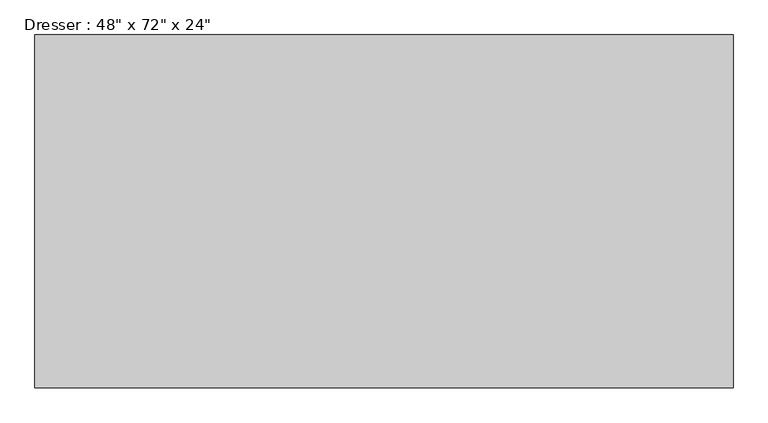
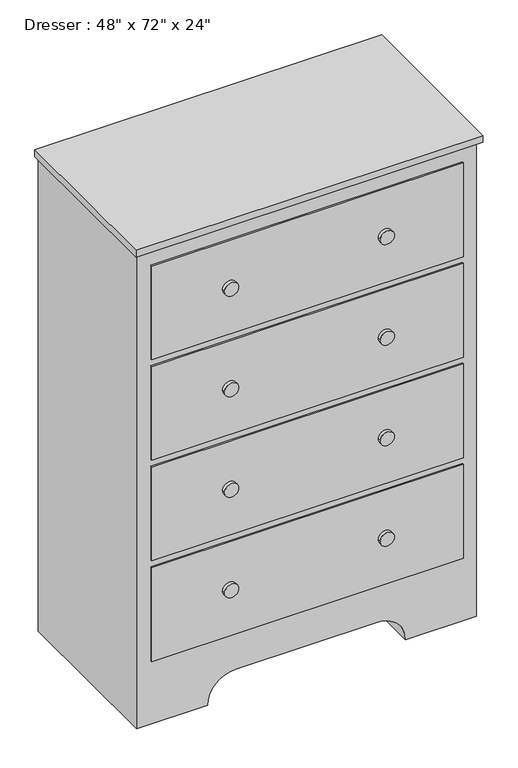
"""IFC4 building model written with IfcOpenShell, lengths in millimetres: furniture geometry."""

from ifc_helpers import new_model, si_unit, point, frame, frame_2d, origin, place, context, project, spatial, polyline, circle_curve, trimmed, segment, composite_curve, outline, extrude, source, transform, mapped, element, save


def furniture_9fa109b2(model_context):
    return source(origin(), model_context, "Body", "SweptSolid", [
        extrude(outline(polyline([(353.1067402, -58.3629541), (353.1067402, -687.0129541), (-891.4932598, -687.0129541), (-891.4932598, -58.3629541), (353.1067402, -58.3629541)])), frame((0.0, 0.0, 1803.4), z_axis=(0.0, 0.0, 1.0), x_axis=(1.0, 0.0, 0.0)), (0.0, 0.0, 1.0), 25.4),
        extrude(outline(composite_curve([segment(polyline([(0.0, 340.4067402), (1803.4, 340.4067402), (1803.4, -878.7932598), (0.0, -878.7932598), (0.0, -624.7932598)]), True, "CONTINUOUS"), segment(trimmed(circle_curve(frame_2d((0.0, -523.1932598)), 101.6), [point((0.0, -624.7932598))], [point((101.6, -523.1932598))], True, "CARTESIAN"), True, "CONTINUOUS"), segment(polyline([(101.6, -523.1932598), (101.6, -15.1932598)]), True, "CONTINUOUS"), segment(trimmed(circle_curve(frame_2d((0.0, -15.1932598)), 101.6), [point((101.6, -15.1932598))], [point((0.0, 86.4067402))], True, "CARTESIAN"), True, "CONTINUOUS"), segment(polyline([(0.0, 86.4067402), (0.0, 340.4067402)]), True, "CONTINUOUS")], self_intersect=False)), frame((0.0, -667.9629541, 0.0), z_axis=(0.0, 1.0, 0.0), x_axis=(0.0, 0.0, 1.0)), (0.0, 0.0, 1.0), 609.6),
        extrude(outline(composite_curve([segment(trimmed(circle_curve(frame_2d((1562.1, 10.2067402)), 25.4), [point((1562.1, -15.1932598))], [point((1562.1, 35.6067402))], False, "CARTESIAN"), True, "CONTINUOUS"), segment(trimmed(circle_curve(frame_2d((1562.1, 10.2067402)), 25.4), [point((1562.1, 35.6067402))], [point((1562.1, -15.1932598))], False, "CARTESIAN"), True, "CONTINUOUS")], self_intersect=False)), frame((0.0, -687.0129541, 0.0), z_axis=(0.0, 1.0, 0.0), x_axis=(0.0, 0.0, 1.0)), (0.0, 0.0, 1.0), 12.7),
        extrude(outline(composite_curve([segment(trimmed(circle_curve(frame_2d((1181.1, 10.2067402)), 25.4), [point((1181.1, -15.1932598))], [point((1181.1, 35.6067402))], False, "CARTESIAN"), True, "CONTINUOUS"), segment(trimmed(circle_curve(frame_2d((1181.1, 10.2067402)), 25.4), [point((1181.1, 35.6067402))], [point((1181.1, -15.1932598))], False, "CARTESIAN"), True, "CONTINUOUS")], self_intersect=False)), frame((0.0, -687.0129541, 0.0), z_axis=(0.0, 1.0, 0.0), x_axis=(0.0, 0.0, 1.0)), (0.0, 0.0, 1.0), 12.7),
        extrude(outline(composite_curve([segment(trimmed(circle_curve(frame_2d((800.1, 10.2067402)), 25.4), [point((800.1, -15.1932598))], [point((800.1, 35.6067402))], False, "CARTESIAN"), True, "CONTINUOUS"), segment(trimmed(circle_curve(frame_2d((800.1, 10.2067402)), 25.4), [point((800.1, 35.6067402))], [point((800.1, -15.1932598))], False, "CARTESIAN"), True, "CONTINUOUS")], self_intersect=False)), frame((0.0, -687.0129541, 0.0), z_axis=(0.0, 1.0, 0.0), x_axis=(0.0, 0.0, 1.0)), (0.0, 0.0, 1.0), 12.7),
        extrude(outline(composite_curve([segment(trimmed(circle_curve(frame_2d((419.1, 10.2067402)), 25.4), [point((419.1, -15.1932598))], [point((419.1, 35.6067402))], False, "CARTESIAN"), True, "CONTINUOUS"), segment(trimmed(circle_curve(frame_2d((419.1, 10.2067402)), 25.4), [point((419.1, 35.6067402))], [point((419.1, -15.1932598))], False, "CARTESIAN"), True, "CONTINUOUS")], self_intersect=False)), frame((0.0, -687.0129541, 0.0), z_axis=(0.0, 1.0, 0.0), x_axis=(0.0, 0.0, 1.0)), (0.0, 0.0, 1.0), 12.7),
        extrude(outline(composite_curve([segment(trimmed(circle_curve(frame_2d((419.1, -548.5932598)), 25.4), [point((419.1, -573.9932598))], [point((419.1, -523.1932598))], False, "CARTESIAN"), True, "CONTINUOUS"), segment(trimmed(circle_curve(frame_2d((419.1, -548.5932598)), 25.4), [point((419.1, -523.1932598))], [point((419.1, -573.9932598))], False, "CARTESIAN"), True, "CONTINUOUS")], self_intersect=False)), frame((0.0, -687.0129541, 0.0), z_axis=(0.0, 1.0, 0.0), x_axis=(0.0, 0.0, 1.0)), (0.0, 0.0, 1.0), 12.7),
        extrude(outline(composite_curve([segment(trimmed(circle_curve(frame_2d((800.1, -548.5932598)), 25.4), [point((800.1, -573.9932598))], [point((800.1, -523.1932598))], False, "CARTESIAN"), True, "CONTINUOUS"), segment(trimmed(circle_curve(frame_2d((800.1, -548.5932598)), 25.4), [point((800.1, -523.1932598))], [point((800.1, -573.9932598))], False, "CARTESIAN"), True, "CONTINUOUS")], self_intersect=False)), frame((0.0, -687.0129541, 0.0), z_axis=(0.0, 1.0, 0.0), x_axis=(0.0, 0.0, 1.0)), (0.0, 0.0, 1.0), 12.7),
        extrude(outline(composite_curve([segment(trimmed(circle_curve(frame_2d((1181.1, -548.5932598)), 25.4), [point((1181.1, -573.9932598))], [point((1181.1, -523.1932598))], False, "CARTESIAN"), True, "CONTINUOUS"), segment(trimmed(circle_curve(frame_2d((1181.1, -548.5932598)), 25.4), [point((1181.1, -523.1932598))], [point((1181.1, -573.9932598))], False, "CARTESIAN"), True, "CONTINUOUS")], self_intersect=False)), frame((0.0, -687.0129541, 0.0), z_axis=(0.0, 1.0, 0.0), x_axis=(0.0, 0.0, 1.0)), (0.0, 0.0, 1.0), 12.7),
        extrude(outline(composite_curve([segment(trimmed(circle_curve(frame_2d((1562.1, -548.5932598)), 25.4), [point((1562.1, -573.9932598))], [point((1562.1, -523.1932598))], False, "CARTESIAN"), True, "CONTINUOUS"), segment(trimmed(circle_curve(frame_2d((1562.1, -548.5932598)), 25.4), [point((1562.1, -523.1932598))], [point((1562.1, -573.9932598))], False, "CARTESIAN"), True, "CONTINUOUS")], self_intersect=False)), frame((0.0, -687.0129541, 0.0), z_axis=(0.0, 1.0, 0.0), x_axis=(0.0, 0.0, 1.0)), (0.0, 0.0, 1.0), 12.7),
        extrude(outline(polyline([(289.6067402, -674.3129541), (-827.9932598, -674.3129541), (-827.9932598, -667.9629541), (289.6067402, -667.9629541), (289.6067402, -674.3129541)])), frame((0.0, 0.0, 1384.3), z_axis=(0.0, 0.0, 1.0), x_axis=(1.0, 0.0, 0.0)), (0.0, 0.0, 1.0), 355.6),
        extrude(outline(polyline([(289.6067402, -674.3129541), (-827.9932598, -674.3129541), (-827.9932598, -667.9629541), (289.6067402, -667.9629541), (289.6067402, -674.3129541)])), frame((0.0, 0.0, 1003.3), z_axis=(0.0, 0.0, 1.0), x_axis=(1.0, 0.0, 0.0)), (0.0, 0.0, 1.0), 355.6),
        extrude(outline(polyline([(289.6067402, -674.3129541), (-827.9932598, -674.3129541), (-827.9932598, -667.9629541), (289.6067402, -667.9629541), (289.6067402, -674.3129541)])), frame((0.0, 0.0, 622.3), z_axis=(0.0, 0.0, 1.0), x_axis=(1.0, 0.0, 0.0)), (0.0, 0.0, 1.0), 355.6),
        extrude(outline(polyline([(289.6067402, -674.3129541), (-827.9932598, -674.3129541), (-827.9932598, -667.9629541), (289.6067402, -667.9629541), (289.6067402, -674.3129541)])), frame((0.0, 0.0, 241.3), z_axis=(0.0, 0.0, 1.0), x_axis=(1.0, 0.0, 0.0)), (0.0, 0.0, 1.0), 355.6),
    ])


if __name__ == "__main__":
    model = new_model("IFC4")
    model_context = context("Model", 3, world=origin())
    ifc_project = project(units=[si_unit("LENGTHUNIT", "METRE", prefix="MILLI")], contexts=[model_context])
    site = spatial("IfcSite", under=ifc_project)
    building = spatial("IfcBuilding", under=site)
    placement = place(None, origin())
    furniture_shape = furniture_9fa109b2(model_context)
    element("IfcFurniture", 1, ObjectType="Dresser : 48\" x 72\" x 24\"", at=placement, inside=building, context=model_context, shape_type="MappedRepresentation", body=[
        mapped(furniture_shape, transform((0.0, 0.0, 0.0), x_axis=(1.0, 0.0, 0.0), y_axis=(0.0, 1.0, 0.0), z_axis=(0.0, 0.0, 1.0))),
    ])
    save(model, "model.ifc")

# Revit data of these elements
# Type "Dresser : 48\" x 72\" x 24\""
#   Assembly Code = "E2020200"
#   Depth = 2' - 0"
#   Height = 6' - 0"
#   Width = 4' - 0"
#   Dresser Material = Wood - Teak
#   Drawer Material = Wood - Teak
#   Knob Material = Cherry
#   Default Elevation = 0
# Element 1 (IfcFurniture, "Dresser : 48\" x 72\" x 24\"")
#   Materials on its faces: "Laminate, Ivory, Matte", "Cherry", "Wood - Teak"
# Materials
#   "Wood - Teak": class "Wood", colour RGB 145 112 90, transparency 0
#   "Cherry": class "Wood", colour RGB 226 177 128, transparency 0, Description = "Prunus Serotina", Cost = 0
#   "Laminate, Ivory, Matte": class "Plastic", colour RGB 247 247 239, transparency 0, Description = "Plastic Laminate - Ivory, Matte", Cost = 0
